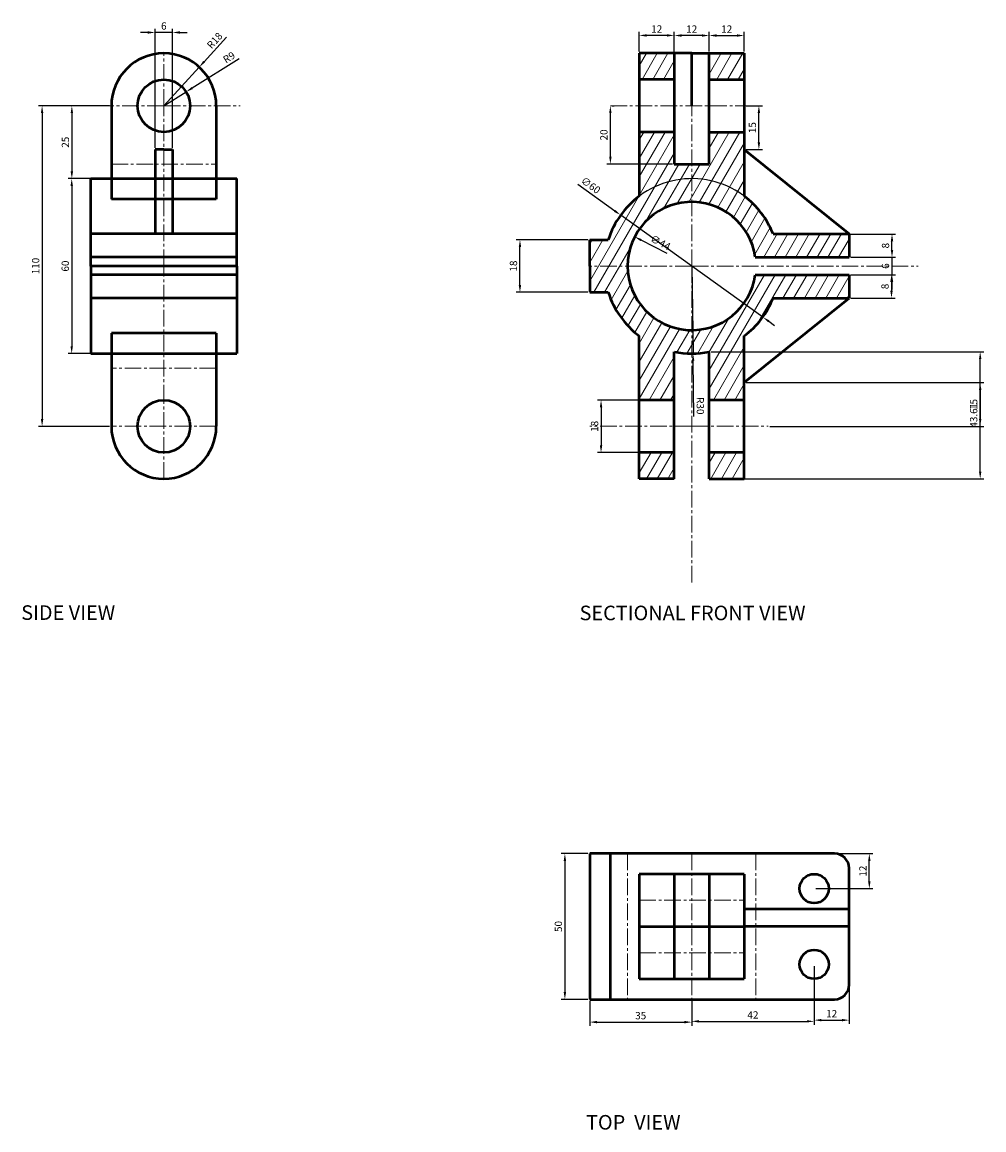
# Model space of a CAD drawing. Units: millimetres. Extents: x 2364 to 2785, y 1000 to 1694.
# Tile 1 of 2: x 2450 to 2780, y 1000 to 1380. Entities that reach past the tile are written whole.
import ezdxf

# ---------------------------------------------------------------- set-up
doc = ezdxf.new("R2010")
doc.units = ezdxf.units.MM
doc.linetypes.add('CENTER2', pattern=[28.575, 19.05, -3.175, 3.175, -3.175])
for name, color, linetype, lineweight in [('M-CNTR', 1, 'CENTER2', 18), ('M-DIMS', 2, 'Continuous', 25), ('M-HATC', 8, 'Continuous', 18), ('M-OUTL', 7, 'Continuous', 50), ('M-TEXT', 3, 'Continuous', 25)]:
    doc.layers.add(name, color=color, linetype=linetype, lineweight=lineweight)
doc.styles.get("Standard").update_dxf_attribs({"font": 'arial.ttf'})
doc.dimstyles.new('ISO-25', dxfattribs={"dimtxt": 2.5, "dimasz": 2.5, "dimexe": 1.25, "dimexo": 0.625, "dimtad": 1, "dimtxsty": 'Standard', "dimcen": 2.5, "dimadec": 0, "dimazin": 0, "dimtfac": 1, "dimtmove": 0, "dimatfit": 3, "dimfxl": 1, "dimarcsym": 0})

# ---------------------------------------------------------------- blocks, each defined once
blk = doc.blocks.new('*D17')
at = {"layer": 'Defpoints', "color": 0, "transparency": 16777216}
for p in [(2697.55, 1375.5), (2685.55, 1369.38), (2697.55, 1369.38)]:
    blk.add_point(p, dxfattribs=at)
at = {"layer": 'M-DIMS', "color": 0, "lineweight": -2, "transparency": 16777216}
for p, q in [((2685.55, 1370.01), (2685.55, 1376.75)), ((2697.55, 1370.01), (2697.55, 1376.75)), ((2688.05, 1375.5), (2695.05, 1375.5))]:
    blk.add_line(p, q, dxfattribs=at)
at = {"layer": 'M-DIMS', "color": 0, "transparency": 16777216}
for points in [[(2688.05, 1375.91), (2688.05, 1375.08), (2685.55, 1375.5)], [(2695.05, 1375.91), (2695.05, 1375.08), (2697.55, 1375.5)]]:
    blk.add_solid(points, dxfattribs=at)
at = {"layer": 'M-DIMS', "color": 0, "transparency": 16777216, "insert": (2691.55, 1377.38), "char_height": 2.5, "attachment_point": 5}
blk.add_mtext('12', dxfattribs=at)
blk = doc.blocks.new('*D18')
at = {"layer": 'Defpoints', "color": 0, "transparency": 16777216}
for p in [(2673.55, 1375.5), (2685.55, 1375.5), (2673.55, 1369.38)]:
    blk.add_point(p, dxfattribs=at)
at = {"layer": 'M-DIMS', "color": 0, "lineweight": -2, "transparency": 16777216}
for p, q in [((2673.55, 1370.01), (2673.55, 1376.75)), ((2685.55, 1376.12), (2685.55, 1376.75)), ((2683.05, 1375.5), (2676.05, 1375.5))]:
    blk.add_line(p, q, dxfattribs=at)
at = {"layer": 'M-DIMS', "color": 0, "transparency": 16777216}
for points in [[(2676.05, 1375.91), (2676.05, 1375.08), (2673.55, 1375.5)], [(2683.05, 1375.91), (2683.05, 1375.08), (2685.55, 1375.5)]]:
    blk.add_solid(points, dxfattribs=at)
at = {"layer": 'M-DIMS', "color": 0, "transparency": 16777216, "insert": (2679.55, 1377.38), "char_height": 2.5, "attachment_point": 5}
blk.add_mtext('12', dxfattribs=at)
blk = doc.blocks.new('*D19')
at = {"layer": 'Defpoints', "color": 0, "transparency": 16777216}
for p in [(2661.55, 1375.53), (2661.55, 1369.38), (2673.55, 1369.38)]:
    blk.add_point(p, dxfattribs=at)
at = {"layer": 'M-DIMS', "color": 0, "lineweight": -2, "transparency": 16777216}
for p, q in [((2661.55, 1370.01), (2661.55, 1376.78)), ((2673.55, 1370.01), (2673.55, 1376.78)), ((2671.05, 1375.53), (2664.05, 1375.53))]:
    blk.add_line(p, q, dxfattribs=at)
at = {"layer": 'M-DIMS', "color": 0, "transparency": 16777216}
for points in [[(2664.05, 1375.94), (2664.05, 1375.11), (2661.55, 1375.53)], [(2671.05, 1375.94), (2671.05, 1375.11), (2673.55, 1375.53)]]:
    blk.add_solid(points, dxfattribs=at)
at = {"layer": 'M-DIMS', "color": 0, "transparency": 16777216, "insert": (2667.55, 1377.41), "char_height": 2.5, "attachment_point": 5}
blk.add_mtext('12', dxfattribs=at)
blk = doc.blocks.new('*D20')
at = {"layer": 'Defpoints', "color": 0, "transparency": 16777216}
for p in [(2651.65, 1351.38), (2651.65, 1351.38), (2673.55, 1331.38)]:
    blk.add_point(p, dxfattribs=at)
at = {"layer": 'M-DIMS', "color": 0, "lineweight": -2, "transparency": 16777216}
for p, q in [((2652.27, 1351.38), (2652.9, 1351.38)), ((2651.65, 1333.88), (2651.65, 1348.88)), ((2672.93, 1331.38), (2650.4, 1331.38))]:
    blk.add_line(p, q, dxfattribs=at)
at = {"layer": 'M-DIMS', "color": 0, "transparency": 16777216}
for points in [[(2651.23, 1348.88), (2652.06, 1348.88), (2651.65, 1351.38)], [(2651.23, 1333.88), (2652.06, 1333.88), (2651.65, 1331.38)]]:
    blk.add_solid(points, dxfattribs=at)
at = {"layer": 'M-DIMS', "color": 0, "transparency": 16777216, "insert": (2649.74, 1341.38), "char_height": 2.5, "attachment_point": 5, "rotation": 90}
blk.add_mtext('20', dxfattribs=at)
blk = doc.blocks.new('*D21')
at = {"layer": 'Defpoints', "color": 0, "transparency": 16777216}
for p in [(2748.25, 1299.38), (2733.55, 1293.38), (2748.25, 1293.38)]:
    blk.add_point(p, dxfattribs=at)
at = {"layer": 'M-DIMS', "color": 0, "lineweight": -2, "transparency": 16777216}
for p, q in [((2748.25, 1301.88), (2748.25, 1304.38)), ((2748.25, 1299.38), (2748.25, 1293.38)), ((2748.88, 1299.38), (2749.5, 1299.38)), ((2734.18, 1293.38), (2749.5, 1293.38)), ((2748.25, 1290.88), (2748.25, 1288.38))]:
    blk.add_line(p, q, dxfattribs=at)
at = {"layer": 'M-DIMS', "color": 0, "transparency": 16777216}
for points in [[(2747.84, 1301.88), (2748.67, 1301.88), (2748.25, 1299.38)], [(2747.84, 1290.88), (2748.67, 1290.88), (2748.25, 1293.38)]]:
    blk.add_solid(points, dxfattribs=at)
at = {"layer": 'M-DIMS', "color": 0, "transparency": 16777216, "insert": (2746.35, 1296.38), "char_height": 2.5, "attachment_point": 5, "rotation": 90}
blk.add_mtext('6', dxfattribs=at)
blk = doc.blocks.new('*D22')
at = {"layer": 'Defpoints', "color": 0, "transparency": 16777216}
for p in [(2733.55, 1293.38), (2733.55, 1285.38), (2748.08, 1285.38)]:
    blk.add_point(p, dxfattribs=at)
at = {"layer": 'M-DIMS', "color": 0, "lineweight": -2, "transparency": 16777216}
for p, q in [((2734.18, 1293.38), (2749.33, 1293.38)), ((2748.08, 1290.88), (2748.08, 1287.88)), ((2734.18, 1285.38), (2749.33, 1285.38))]:
    blk.add_line(p, q, dxfattribs=at)
at = {"layer": 'M-DIMS', "color": 0, "transparency": 16777216}
for points in [[(2747.66, 1290.88), (2748.49, 1290.88), (2748.08, 1293.38)], [(2747.66, 1287.88), (2748.49, 1287.88), (2748.08, 1285.38)]]:
    blk.add_solid(points, dxfattribs=at)
at = {"layer": 'M-DIMS', "color": 0, "transparency": 16777216, "insert": (2746.18, 1289.38), "char_height": 2.5, "attachment_point": 5, "rotation": 90}
blk.add_mtext('8', dxfattribs=at)
blk = doc.blocks.new('*D23')
at = {"layer": 'Defpoints', "color": 0, "transparency": 16777216}
for p in [(2659.98, 1306.43), (2699.13, 1286.34)]:
    blk.add_point(p, dxfattribs=at)
at = {"layer": 'M-DIMS', "color": 0, "lineweight": -2, "transparency": 16777216}
blk.add_line((2671.14, 1300.7), (2662.2, 1305.29), dxfattribs=at)
at = {"layer": 'M-DIMS', "color": 0, "transparency": 16777216}
blk.add_solid([(2662.39, 1305.66), (2662.01, 1304.92), (2659.98, 1306.43)], dxfattribs=at)
at = {"layer": 'M-DIMS', "color": 0, "transparency": 16777216, "insert": (2668.68, 1304.18), "char_height": 2.5, "attachment_point": 5, "rotation": 332.8312}
blk.add_mtext('∅44', dxfattribs=at)
blk = doc.blocks.new('*D24')
at = {"layer": 'Defpoints', "color": 0, "transparency": 16777216}
for p in [(2655.18, 1313.88), (2703.92, 1278.89)]:
    blk.add_point(p, dxfattribs=at)
at = {"layer": 'M-DIMS', "color": 0, "lineweight": -2, "transparency": 16777216}
for p, q in [((2640.48, 1324.44), (2653.15, 1315.34)), ((2703.92, 1278.89), (2655.18, 1313.88)), ((2705.95, 1277.43), (2707.98, 1275.97))]:
    blk.add_line(p, q, dxfattribs=at)
blk.add_arc((2679.55, 1296.38), 30, 54.3238, 146.7095, dxfattribs=at)
at = {"layer": 'M-DIMS', "color": 0, "transparency": 16777216}
for points in [[(2653.4, 1315.68), (2652.91, 1315), (2655.18, 1313.88)], [(2706.2, 1277.77), (2705.71, 1277.09), (2703.92, 1278.89)]]:
    blk.add_solid(points, dxfattribs=at)
at = {"layer": 'M-DIMS', "color": 0, "transparency": 16777216, "insert": (2644.7, 1323.84), "char_height": 2.5, "attachment_point": 5, "rotation": 324.3222}
blk.add_mtext('∅60', dxfattribs=at)
blk = doc.blocks.new('*D25')
at = {"layer": 'Defpoints', "color": 0, "transparency": 16777216}
for p in [(2661.55, 1250.38), (2648.45, 1232.38), (2661.55, 1232.38)]:
    blk.add_point(p, dxfattribs=at)
at = {"layer": 'M-DIMS', "color": 0, "lineweight": -2, "transparency": 16777216}
for p, q in [((2660.93, 1250.38), (2647.2, 1250.38)), ((2648.45, 1247.88), (2648.45, 1234.88)), ((2660.93, 1232.38), (2647.2, 1232.38))]:
    blk.add_line(p, q, dxfattribs=at)
at = {"layer": 'M-DIMS', "color": 0, "transparency": 16777216}
for points in [[(2648.03, 1247.88), (2648.87, 1247.88), (2648.45, 1250.38)], [(2648.03, 1234.88), (2648.87, 1234.88), (2648.45, 1232.38)]]:
    blk.add_solid(points, dxfattribs=at)
at = {"layer": 'M-DIMS', "color": 0, "transparency": 16777216, "insert": (2646.55, 1241.38), "char_height": 2.5, "attachment_point": 5, "rotation": 90}
blk.add_mtext('18', dxfattribs=at)
blk = doc.blocks.new('*D26')
at = {"layer": 'Defpoints', "color": 0, "transparency": 16777216}
for p in [(2620.63, 1305.38), (2644.55, 1305.38), (2644.55, 1287.38)]:
    blk.add_point(p, dxfattribs=at)
at = {"layer": 'M-DIMS', "color": 0, "lineweight": -2, "transparency": 16777216}
for p, q in [((2643.93, 1305.38), (2619.38, 1305.38)), ((2620.63, 1289.88), (2620.63, 1302.88)), ((2643.93, 1287.38), (2619.38, 1287.38))]:
    blk.add_line(p, q, dxfattribs=at)
at = {"layer": 'M-DIMS', "color": 0, "transparency": 16777216}
for points in [[(2620.21, 1302.88), (2621.05, 1302.88), (2620.63, 1305.38)], [(2620.21, 1289.88), (2621.05, 1289.88), (2620.63, 1287.38)]]:
    blk.add_solid(points, dxfattribs=at)
at = {"layer": 'M-DIMS', "color": 0, "transparency": 16777216, "insert": (2618.73, 1296.38), "char_height": 2.5, "attachment_point": 5, "rotation": 90}
blk.add_mtext('18', dxfattribs=at)
blk = doc.blocks.new('*D27')
at = {"layer": 'Defpoints', "color": 0, "transparency": 16777216}
for p in [(2733.55, 1307.38), (2748.25, 1307.38), (2733.55, 1299.38)]:
    blk.add_point(p, dxfattribs=at)
at = {"layer": 'M-DIMS', "color": 0, "lineweight": -2, "transparency": 16777216}
for p, q in [((2734.18, 1307.38), (2749.5, 1307.38)), ((2748.25, 1301.88), (2748.25, 1304.88)), ((2734.18, 1299.38), (2749.5, 1299.38))]:
    blk.add_line(p, q, dxfattribs=at)
at = {"layer": 'M-DIMS', "color": 0, "transparency": 16777216}
for points in [[(2747.84, 1304.88), (2748.67, 1304.88), (2748.25, 1307.38)], [(2747.84, 1301.88), (2748.67, 1301.88), (2748.25, 1299.38)]]:
    blk.add_solid(points, dxfattribs=at)
at = {"layer": 'M-DIMS', "color": 0, "transparency": 16777216, "insert": (2746.35, 1303.38), "char_height": 2.5, "attachment_point": 5, "rotation": 90}
blk.add_mtext('8', dxfattribs=at)
blk = doc.blocks.new('*D28')
at = {"layer": 'Defpoints', "color": 0, "transparency": 16777216}
for p in [(2697.55, 1351.38), (2702.59, 1351.38), (2697.55, 1336.38)]:
    blk.add_point(p, dxfattribs=at)
at = {"layer": 'M-DIMS', "color": 0, "lineweight": -2, "transparency": 16777216}
for p, q in [((2698.18, 1351.38), (2703.84, 1351.38)), ((2702.59, 1338.88), (2702.59, 1348.88)), ((2698.18, 1336.38), (2703.84, 1336.38))]:
    blk.add_line(p, q, dxfattribs=at)
at = {"layer": 'M-DIMS', "color": 0, "transparency": 16777216}
for points in [[(2702.17, 1348.88), (2703.01, 1348.88), (2702.59, 1351.38)], [(2702.17, 1338.88), (2703.01, 1338.88), (2702.59, 1336.38)]]:
    blk.add_solid(points, dxfattribs=at)
at = {"layer": 'M-DIMS', "color": 0, "transparency": 16777216, "insert": (2700.69, 1343.88), "char_height": 2.5, "attachment_point": 5, "rotation": 90}
blk.add_mtext('15', dxfattribs=at)
blk = doc.blocks.new('*D29')
at = {"layer": 'Defpoints', "color": 0, "transparency": 16777216}
for p in [(2480.47, 1351.38), (2466.92, 1326.38), (2480.47, 1326.38)]:
    blk.add_point(p, dxfattribs=at)
at = {"layer": 'M-DIMS', "color": 0, "lineweight": -2, "transparency": 16777216}
for p, q in [((2479.84, 1351.38), (2465.67, 1351.38)), ((2466.92, 1348.88), (2466.92, 1328.88)), ((2479.84, 1326.38), (2465.67, 1326.38))]:
    blk.add_line(p, q, dxfattribs=at)
at = {"layer": 'M-DIMS', "color": 0, "transparency": 16777216}
for points in [[(2466.5, 1348.88), (2467.33, 1348.88), (2466.92, 1351.38)], [(2466.5, 1328.88), (2467.33, 1328.88), (2466.92, 1326.38)]]:
    blk.add_solid(points, dxfattribs=at)
at = {"layer": 'M-DIMS', "color": 0, "transparency": 16777216, "insert": (2465.02, 1338.88), "char_height": 2.5, "attachment_point": 5, "rotation": 90}
blk.add_mtext('25', dxfattribs=at)
blk = doc.blocks.new('*D30')
at = {"layer": 'Defpoints', "color": 0, "transparency": 16777216}
for p in [(2480.47, 1351.38), (2456.71, 1241.38), (2480.47, 1241.38)]:
    blk.add_point(p, dxfattribs=at)
at = {"layer": 'M-DIMS', "color": 0, "lineweight": -2, "transparency": 16777216}
for p, q in [((2479.84, 1351.38), (2455.46, 1351.38)), ((2456.71, 1348.88), (2456.71, 1243.88)), ((2479.84, 1241.38), (2455.46, 1241.38))]:
    blk.add_line(p, q, dxfattribs=at)
at = {"layer": 'M-DIMS', "color": 0, "transparency": 16777216}
for points in [[(2456.29, 1348.88), (2457.13, 1348.88), (2456.71, 1351.38)], [(2456.29, 1243.88), (2457.13, 1243.88), (2456.71, 1241.38)]]:
    blk.add_solid(points, dxfattribs=at)
at = {"layer": 'M-DIMS', "color": 0, "transparency": 16777216, "insert": (2454.81, 1296.38), "char_height": 2.5, "attachment_point": 5, "rotation": 90}
blk.add_mtext('110', dxfattribs=at)
blk = doc.blocks.new('*D31')
at = {"layer": 'Defpoints', "color": 0, "transparency": 16777216}
for p in [(2480.47, 1326.38), (2466.87, 1266.38), (2480.47, 1266.38)]:
    blk.add_point(p, dxfattribs=at)
at = {"layer": 'M-DIMS', "color": 0, "lineweight": -2, "transparency": 16777216}
for p, q in [((2479.84, 1326.38), (2465.62, 1326.38)), ((2466.87, 1323.88), (2466.87, 1268.88)), ((2479.84, 1266.38), (2465.62, 1266.38))]:
    blk.add_line(p, q, dxfattribs=at)
at = {"layer": 'M-DIMS', "color": 0, "transparency": 16777216}
for points in [[(2466.45, 1323.88), (2467.29, 1323.88), (2466.87, 1326.38)], [(2466.45, 1268.88), (2467.29, 1268.88), (2466.87, 1266.38)]]:
    blk.add_solid(points, dxfattribs=at)
at = {"layer": 'M-DIMS', "color": 0, "transparency": 16777216, "insert": (2464.97, 1296.38), "char_height": 2.5, "attachment_point": 5, "rotation": 90}
blk.add_mtext('60', dxfattribs=at)
blk = doc.blocks.new('*D32')
at = {"layer": 'Defpoints', "color": 0, "transparency": 16777216}
for p in [(2495.47, 1376.54), (2495.47, 1336.38), (2501.47, 1336.38)]:
    blk.add_point(p, dxfattribs=at)
at = {"layer": 'M-DIMS', "color": 0, "lineweight": -2, "transparency": 16777216}
for p, q in [((2492.97, 1376.54), (2490.47, 1376.54)), ((2495.47, 1337.01), (2495.47, 1377.79)), ((2501.47, 1376.54), (2495.47, 1376.54)), ((2501.47, 1337.01), (2501.47, 1377.79)), ((2503.97, 1376.54), (2506.47, 1376.54))]:
    blk.add_line(p, q, dxfattribs=at)
at = {"layer": 'M-DIMS', "color": 0, "transparency": 16777216}
for points in [[(2492.97, 1376.96), (2492.97, 1376.12), (2495.47, 1376.54)], [(2503.97, 1376.96), (2503.97, 1376.12), (2501.47, 1376.54)]]:
    blk.add_solid(points, dxfattribs=at)
at = {"layer": 'M-DIMS', "color": 0, "transparency": 16777216, "insert": (2498.47, 1378.44), "char_height": 2.5, "attachment_point": 5}
blk.add_mtext('6', dxfattribs=at)
blk = doc.blocks.new('*D33')
at = {"layer": 'Defpoints', "color": 0, "transparency": 16777216}
for p in [(2510.61, 1364.68), (2498.47, 1351.38)]:
    blk.add_point(p, dxfattribs=at)
at = {"layer": 'M-DIMS', "color": 0, "lineweight": -2, "transparency": 16777216}
for p, q in [((2519.99, 1374.95), (2512.29, 1366.52)), ((2498.47, 1351.38), (2510.61, 1364.68))]:
    blk.add_line(p, q, dxfattribs=at)
at = {"layer": 'M-DIMS', "color": 0, "transparency": 16777216}
blk.add_solid([(2511.99, 1366.8), (2512.6, 1366.24), (2510.61, 1364.68)], dxfattribs=at)
at = {"layer": 'M-DIMS', "color": 0, "transparency": 16777216, "insert": (2516.15, 1373.56), "char_height": 2.5, "attachment_point": 5, "rotation": 47.5926}
blk.add_mtext('R18', dxfattribs=at)
blk = doc.blocks.new('*D34')
at = {"layer": 'Defpoints', "color": 0, "transparency": 16777216}
for p in [(2506.1, 1356.16), (2498.47, 1351.38)]:
    blk.add_point(p, dxfattribs=at)
at = {"layer": 'M-DIMS', "color": 0, "lineweight": -2, "transparency": 16777216}
for p, q in [((2524.26, 1367.51), (2508.22, 1357.48)), ((2498.47, 1351.38), (2506.1, 1356.16))]:
    blk.add_line(p, q, dxfattribs=at)
at = {"layer": 'M-DIMS', "color": 0, "transparency": 16777216}
blk.add_solid([(2508, 1357.83), (2508.44, 1357.13), (2506.1, 1356.16)], dxfattribs=at)
at = {"layer": 'M-DIMS', "color": 0, "transparency": 16777216, "insert": (2521.01, 1367.72), "char_height": 2.5, "attachment_point": 5, "rotation": 32.0078}
blk.add_mtext('R9', dxfattribs=at)
blk = doc.blocks.new('*D35')
at = {"layer": 'Defpoints', "color": 0, "transparency": 16777216}
for p in [(2721.55, 1094.74), (2740.47, 1094.74), (2721.55, 1082.74)]:
    blk.add_point(p, dxfattribs=at)
at = {"layer": 'M-DIMS', "color": 0, "lineweight": -2, "transparency": 16777216}
for p, q in [((2722.18, 1094.74), (2741.72, 1094.74)), ((2740.47, 1085.24), (2740.47, 1092.24)), ((2722.18, 1082.74), (2741.72, 1082.74))]:
    blk.add_line(p, q, dxfattribs=at)
at = {"layer": 'M-DIMS', "color": 0, "transparency": 16777216}
for points in [[(2740.06, 1092.24), (2740.89, 1092.24), (2740.47, 1094.74)], [(2740.06, 1085.24), (2740.89, 1085.24), (2740.47, 1082.74)]]:
    blk.add_solid(points, dxfattribs=at)
at = {"layer": 'M-DIMS', "color": 0, "transparency": 16777216, "insert": (2738.59, 1088.74), "char_height": 2.5, "attachment_point": 5, "rotation": 90}
blk.add_mtext('12', dxfattribs=at)
blk = doc.blocks.new('*D36')
at = {"layer": 'Defpoints', "color": 0, "transparency": 16777216}
for p in [(2644.55, 1094.74), (2636.04, 1044.74), (2644.55, 1044.74)]:
    blk.add_point(p, dxfattribs=at)
at = {"layer": 'M-DIMS', "color": 0, "lineweight": -2, "transparency": 16777216}
for p, q in [((2643.93, 1094.74), (2634.79, 1094.74)), ((2636.04, 1092.24), (2636.04, 1047.24)), ((2643.93, 1044.74), (2634.79, 1044.74))]:
    blk.add_line(p, q, dxfattribs=at)
at = {"layer": 'M-DIMS', "color": 0, "transparency": 16777216}
for points in [[(2635.62, 1092.24), (2636.46, 1092.24), (2636.04, 1094.74)], [(2635.62, 1047.24), (2636.46, 1047.24), (2636.04, 1044.74)]]:
    blk.add_solid(points, dxfattribs=at)
at = {"layer": 'M-DIMS', "color": 0, "transparency": 16777216, "insert": (2634.14, 1069.74), "char_height": 2.5, "attachment_point": 5, "rotation": 90}
blk.add_mtext('50', dxfattribs=at)
blk = doc.blocks.new('*D37')
at = {"layer": 'Defpoints', "color": 0, "transparency": 16777216}
for p in [(2644.55, 1044.74), (2679.55, 1044.74), (2679.55, 1036.92)]:
    blk.add_point(p, dxfattribs=at)
at = {"layer": 'M-DIMS', "color": 0, "lineweight": -2, "transparency": 16777216}
for p, q in [((2644.55, 1044.12), (2644.55, 1035.67)), ((2679.55, 1044.12), (2679.55, 1035.67)), ((2647.05, 1036.92), (2677.05, 1036.92))]:
    blk.add_line(p, q, dxfattribs=at)
at = {"layer": 'M-DIMS', "color": 0, "transparency": 16777216}
for points in [[(2647.05, 1037.34), (2647.05, 1036.5), (2644.55, 1036.92)], [(2677.05, 1037.34), (2677.05, 1036.5), (2679.55, 1036.92)]]:
    blk.add_solid(points, dxfattribs=at)
at = {"layer": 'M-DIMS', "color": 0, "transparency": 16777216, "insert": (2662.05, 1038.82), "char_height": 2.5, "attachment_point": 5}
blk.add_mtext('35', dxfattribs=at)
blk = doc.blocks.new('*D38')
at = {"layer": 'Defpoints', "color": 0, "transparency": 16777216}
for p in [(2721.55, 1056.74), (2679.55, 1044.74), (2721.55, 1037.19)]:
    blk.add_point(p, dxfattribs=at)
at = {"layer": 'M-DIMS', "color": 0, "lineweight": -2, "transparency": 16777216}
for p, q in [((2721.55, 1056.12), (2721.55, 1035.94)), ((2679.55, 1044.12), (2679.55, 1035.94)), ((2682.05, 1037.19), (2719.05, 1037.19))]:
    blk.add_line(p, q, dxfattribs=at)
at = {"layer": 'M-DIMS', "color": 0, "transparency": 16777216}
for points in [[(2682.05, 1037.61), (2682.05, 1036.78), (2679.55, 1037.19)], [(2719.05, 1037.61), (2719.05, 1036.78), (2721.55, 1037.19)]]:
    blk.add_solid(points, dxfattribs=at)
at = {"layer": 'M-DIMS', "color": 0, "transparency": 16777216, "insert": (2700.55, 1039.07), "char_height": 2.5, "attachment_point": 5}
blk.add_mtext('42', dxfattribs=at)
blk = doc.blocks.new('*D39')
at = {"layer": 'Defpoints', "color": 0, "transparency": 16777216}
for p in [(2721.55, 1056.74), (2733.55, 1056.74), (2733.55, 1037.61)]:
    blk.add_point(p, dxfattribs=at)
at = {"layer": 'M-DIMS', "color": 0, "lineweight": -2, "transparency": 16777216}
for p, q in [((2721.55, 1056.12), (2721.55, 1036.36)), ((2733.55, 1056.12), (2733.55, 1036.36)), ((2724.05, 1037.61), (2731.05, 1037.61))]:
    blk.add_line(p, q, dxfattribs=at)
at = {"layer": 'M-DIMS', "color": 0, "transparency": 16777216}
for points in [[(2724.05, 1038.02), (2724.05, 1037.19), (2721.55, 1037.61)], [(2731.05, 1038.02), (2731.05, 1037.19), (2733.55, 1037.61)]]:
    blk.add_solid(points, dxfattribs=at)
at = {"layer": 'M-DIMS', "color": 0, "transparency": 16777216, "insert": (2727.55, 1039.49), "char_height": 2.5, "attachment_point": 5}
blk.add_mtext('12', dxfattribs=at)
blk = doc.blocks.new('*D40')
at = {"layer": 'Defpoints', "color": 0, "transparency": 16777216}
for p in [(2685.55, 1266.99), (2778.5, 1266.99), (2685.55, 1223.38)]:
    blk.add_point(p, dxfattribs=at)
at = {"layer": 'M-DIMS', "color": 0, "lineweight": -2, "transparency": 16777216}
for p, q in [((2686.18, 1266.99), (2779.75, 1266.99)), ((2778.5, 1225.88), (2778.5, 1264.49)), ((2686.18, 1223.38), (2779.75, 1223.38))]:
    blk.add_line(p, q, dxfattribs=at)
at = {"layer": 'M-DIMS', "color": 0, "transparency": 16777216}
for points in [[(2778.09, 1264.49), (2778.92, 1264.49), (2778.5, 1266.99)], [(2778.09, 1225.88), (2778.92, 1225.88), (2778.5, 1223.38)]]:
    blk.add_solid(points, dxfattribs=at)
at = {"layer": 'M-DIMS', "color": 0, "transparency": 16777216, "insert": (2776.6, 1245.19), "char_height": 2.5, "attachment_point": 5, "rotation": 90}
blk.add_mtext('43.61', dxfattribs=at)
blk = doc.blocks.new('*D41')
at = {"layer": 'Defpoints', "color": 0, "transparency": 16777216}
for p in [(2697.55, 1256.38), (2705.76, 1241.38), (2778.5, 1241.38)]:
    blk.add_point(p, dxfattribs=at)
at = {"layer": 'M-DIMS', "color": 0, "lineweight": -2, "transparency": 16777216}
for p, q in [((2698.18, 1256.38), (2779.75, 1256.38)), ((2778.5, 1253.88), (2778.5, 1243.88)), ((2706.39, 1241.38), (2779.75, 1241.38))]:
    blk.add_line(p, q, dxfattribs=at)
at = {"layer": 'M-DIMS', "color": 0, "transparency": 16777216}
for points in [[(2778.09, 1253.88), (2778.92, 1253.88), (2778.5, 1256.38)], [(2778.09, 1243.88), (2778.92, 1243.88), (2778.5, 1241.38)]]:
    blk.add_solid(points, dxfattribs=at)
at = {"layer": 'M-DIMS', "color": 0, "transparency": 16777216, "insert": (2776.6, 1248.88), "char_height": 2.5, "attachment_point": 5, "rotation": 90}
blk.add_mtext('15', dxfattribs=at)
blk = doc.blocks.new('*D42')
at = {"layer": 'Defpoints', "color": 0, "transparency": 16777216}
for p in [(2679.55, 1296.38), (2680, 1266.39)]:
    blk.add_point(p, dxfattribs=at)
at = {"layer": 'M-DIMS', "color": 0, "lineweight": -2, "transparency": 16777216}
for p, q in [((2679.55, 1296.38), (2680, 1266.39)), ((2680.32, 1244.78), (2680.04, 1263.89))]:
    blk.add_line(p, q, dxfattribs=at)
at = {"layer": 'M-DIMS', "color": 0, "transparency": 16777216}
blk.add_solid([(2680.45, 1263.89), (2679.62, 1263.88), (2680, 1266.39)], dxfattribs=at)
at = {"layer": 'M-DIMS', "color": 0, "transparency": 16777216, "insert": (2682.17, 1248.42), "char_height": 2.5, "attachment_point": 5, "rotation": 270.8551}
blk.add_mtext('R30', dxfattribs=at)

msp = doc.modelspace()

# ---------------------------------------------------------------- hatches: boundary and pattern name
at = {"layer": 'M-HATC'}
h = msp.add_hatch(dxfattribs=at)
h.set_pattern_fill('ANSI31', color=256, angle=15)
h.paths.add_polyline_path([(2679.552, 1331.385), (2673.552, 1331.385), (2673.552, 1342.385), (2661.552, 1342.385), (2661.552, 1320.385, 0.1569199), (2650.934, 1305.385), (2644.552, 1305.385), (2644.552, 1296.385), (2657.552, 1296.385, -0.4142136), (2679.552, 1318.385)])
h.paths.add_polyline_path([(2697.552, 1342.385), (2685.552, 1342.385), (2685.552, 1331.385), (2679.552, 1331.385), (2679.552, 1318.385, -0.3746932), (2701.347, 1299.385), (2733.552, 1299.385), (2733.552, 1307.385), (2707.463, 1307.385, 0.13885), (2697.552, 1320.385)])
h.paths.add_polyline_path([(2697.552, 1272.385, 0.13885), (2707.463, 1285.385), (2733.552, 1285.385), (2733.552, 1293.385), (2701.347, 1293.385, -0.3746932), (2679.552, 1274.385), (2679.552, 1266.385, 0.050382), (2685.552, 1266.991), (2685.552, 1250.385), (2697.552, 1250.385)])
h.paths.add_polyline_path([(2679.552, 1274.385, -0.4142136), (2657.552, 1296.385), (2644.552, 1296.385), (2644.552, 1287.385), (2650.934, 1287.385, 0.1569199), (2661.552, 1272.385), (2661.552, 1250.385), (2673.552, 1250.385), (2673.552, 1266.991, 0.050382), (2679.552, 1266.385)])
h.paths.add_polyline_path([(2673.552, 1232.385), (2661.552, 1232.385), (2661.552, 1223.385), (2673.552, 1223.385)])
h.paths.add_polyline_path([(2697.552, 1232.385), (2685.552, 1232.385), (2685.552, 1223.385), (2697.552, 1223.385)])
h.paths.add_polyline_path([(2673.552, 1369.385), (2661.552, 1369.385), (2661.552, 1360.385), (2673.552, 1360.385)])
h.paths.add_polyline_path([(2697.552, 1369.385), (2685.552, 1369.385), (2685.552, 1360.385), (2697.552, 1360.385)])

# ---------------------------------------------------------------- linework, layer by layer
at = {"layer": 'M-CNTR', "ltscale": 0.3}
for p, q in [((2498.468, 1351.385), (2498.468, 1369.385)), ((2498.468, 1351.385), (2471.755, 1351.385)), ((2498.468, 1296.385), (2498.468, 1351.385)), ((2498.468, 1351.385), (2524.69, 1351.385)), ((2651.646, 1351.385), (2703.004, 1351.385)), ((2679.552, 1296.385), (2679.552, 1351.385)), ((2480.468, 1331.385), (2516.468, 1331.385)), ((2523.468, 1296.385), (2473.468, 1296.385)), ((2498.468, 1249.902), (2498.468, 1296.385)), ((2679.552, 1296.385), (2644.552, 1296.385)), ((2679.552, 1296.385), (2757.254, 1296.385)), ((2679.552, 1296.385), (2679.552, 1187.563)), ((2516.468, 1261.385), (2480.468, 1261.385)), ((2498.468, 1223.385), (2498.468, 1249.902)), ((2516.468, 1241.385), (2480.468, 1241.385)), ((2679.552, 1241.385), (2644.552, 1241.385)), ((2679.552, 1241.385), (2705.762, 1241.385)), ((2657.552, 1094.744), (2657.552, 1044.744)), ((2679.552, 1094.744), (2679.552, 1044.744)), ((2701.552, 1094.744), (2701.552, 1044.744)), ((2661.552, 1078.744), (2697.552, 1078.744)), ((2661.552, 1060.744), (2697.552, 1060.744))]:
    msp.add_line(p, q, dxfattribs=at)
at = {"layer": 'M-OUTL'}
for p, q in [((2673.552, 1369.385), (2661.552, 1369.385)), ((2661.552, 1369.385), (2661.552, 1320.385)), ((2679.552, 1369.385), (2673.552, 1369.385)), ((2673.552, 1369.385), (2673.552, 1351.385)), ((2679.552, 1351.385), (2679.552, 1369.385)), ((2679.552, 1369.385), (2685.552, 1369.385)), ((2685.552, 1369.385), (2697.552, 1369.385)), ((2685.552, 1351.385), (2685.552, 1369.385)), ((2697.552, 1369.385), (2697.552, 1320.385)), ((2673.552, 1360.385), (2661.552, 1360.385)), ((2685.552, 1360.385), (2697.552, 1360.385)), ((2480.468, 1351.385), (2480.468, 1319.385)), ((2516.468, 1351.385), (2516.468, 1319.385)), ((2673.552, 1351.385), (2673.552, 1331.385)), ((2685.552, 1331.385), (2685.552, 1351.385)), ((2673.552, 1342.385), (2661.552, 1342.385)), ((2685.552, 1342.385), (2697.552, 1342.385)), ((2498.468, 1336.385), (2495.468, 1336.385)), ((2495.468, 1336.385), (2495.468, 1307.385)), ((2498.468, 1336.385), (2501.468, 1336.385)), ((2501.468, 1336.385), (2501.468, 1307.385)), ((2697.552, 1336.385), (2733.552, 1307.385)), ((2673.552, 1331.385), (2685.552, 1331.385)), ((2473.468, 1296.385), (2473.468, 1326.385)), ((2473.468, 1326.385), (2523.468, 1326.385)), ((2523.468, 1296.385), (2523.468, 1326.385)), ((2516.468, 1319.385), (2480.468, 1319.385)), ((2523.468, 1307.385), (2473.468, 1307.385)), ((2644.552, 1296.385), (2644.552, 1305.385)), ((2644.552, 1305.385), (2650.934, 1305.385)), ((2707.463, 1307.385), (2733.552, 1307.385)), ((2733.552, 1307.385), (2733.552, 1299.385)), ((2523.468, 1299.385), (2473.468, 1299.385)), ((2473.468, 1296.385), (2473.468, 1266.385)), ((2523.468, 1296.385), (2473.468, 1296.385)), ((2523.468, 1296.385), (2523.468, 1266.385)), ((2644.552, 1296.385), (2644.552, 1287.385)), ((2701.347, 1299.385), (2733.552, 1299.385)), ((2523.468, 1293.385), (2473.468, 1293.385)), ((2701.347, 1293.385), (2733.552, 1293.385)), ((2733.552, 1293.385), (2733.552, 1285.385)), ((2523.468, 1285.385), (2473.468, 1285.385)), ((2644.552, 1287.385), (2650.934, 1287.385)), ((2697.552, 1256.385), (2733.552, 1285.385)), ((2707.463, 1285.385), (2733.552, 1285.385)), ((2516.468, 1273.385), (2480.468, 1273.385)), ((2480.468, 1273.385), (2480.468, 1241.385)), ((2516.468, 1273.385), (2516.468, 1266.385)), ((2661.552, 1223.385), (2661.552, 1272.385)), ((2697.552, 1223.385), (2697.552, 1272.385)), ((2473.468, 1266.385), (2523.468, 1266.385)), ((2516.468, 1266.385), (2516.468, 1241.385)), ((2673.552, 1223.385), (2673.552, 1266.991)), ((2685.552, 1223.385), (2685.552, 1266.991)), ((2673.552, 1250.385), (2661.552, 1250.385)), ((2697.552, 1250.385), (2685.552, 1250.385)), ((2673.552, 1232.385), (2661.552, 1232.385)), ((2697.552, 1232.385), (2685.552, 1232.385)), ((2673.552, 1223.385), (2661.552, 1223.385)), ((2685.552, 1223.385), (2697.552, 1223.385)), ((2728.552, 1094.744), (2644.552, 1094.744)), ((2644.552, 1094.744), (2644.552, 1044.744)), ((2651.552, 1094.744), (2651.552, 1044.744)), ((2661.552, 1087.744), (2661.552, 1051.744)), ((2697.552, 1087.744), (2661.552, 1087.744)), ((2673.552, 1087.744), (2673.552, 1051.744)), ((2685.552, 1087.744), (2685.552, 1051.744)), ((2697.552, 1087.744), (2697.552, 1051.744)), ((2733.552, 1049.744), (2733.552, 1089.744)), ((2733.552, 1075.744), (2697.552, 1075.744)), ((2661.552, 1069.744), (2697.552, 1069.744)), ((2733.552, 1069.744), (2697.552, 1069.744)), ((2661.552, 1051.744), (2697.552, 1051.744)), ((2644.552, 1044.744), (2728.552, 1044.744))]:
    msp.add_line(p, q, dxfattribs=at)
for centre, radius in [((2498.468, 1351.385), 9), ((2498.468, 1241.385), 9), ((2721.552, 1082.744), 5), ((2721.552, 1056.744), 5)]:
    msp.add_circle(centre, radius, dxfattribs=at)
for centre, radius, start, end in [((2498.468, 1351.385), 18, 0, 180), ((2679.552, 1296.385), 30, 126.8699, 162.5424), ((2679.552, 1296.385), 30, 21.51019, 53.1301), ((2679.552, 1296.385), 22, 7.83748, 352.16252), ((2679.552, 1296.385), 30, 197.4576, 233.1301), ((2679.552, 1296.385), 30, 306.8699, 338.48981), ((2679.552, 1296.385), 30, 258.46304, 281.53696), ((2498.468, 1241.385), 18, 180, 0), ((2728.552, 1089.744), 5, 0, 90), ((2728.552, 1049.744), 5, 270, 0)]:
    msp.add_arc(centre, radius, start, end, dxfattribs=at)

# ---------------------------------------------------------------- texts
at = {"layer": 'M-TEXT', "char_height": 5, "attachment_point": 1}
for s, insert in [('SIDE VIEW', (2449.545, 1179.961)), ('SECTIONAL FRONT VIEW', (2641.072, 1179.837)), ('TOP  VIEW', (2643.285, 1005.045))]:
    msp.add_mtext_dynamic_manual_height_columns(s, width=88.56628, gutter_width=12.5, heights=[0], dxfattribs=dict(at, insert=insert))

# ---------------------------------------------------------------- dimensions: what is measured, and where the dimension line sits
at = {"layer": 'M-DIMS'}
for base, p1, p2, picture, middle in [((2495.468, 1376.54), (2501.468, 1336.385), (2495.468, 1336.385), '*D32', (2498.468, 1378.442)), ((2661.552, 1375.526), (2673.552, 1369.385), (2661.552, 1369.385), '*D19', (2667.552, 1377.406)), ((2673.552, 1375.496), (2685.552, 1375.496), (2673.552, 1369.385), '*D18', (2679.552, 1377.376)), ((2697.552, 1375.496), (2685.552, 1369.385), (2697.552, 1369.385), '*D17', (2691.552, 1377.376)), ((2721.552, 1037.195), (2679.552, 1044.744), (2721.552, 1056.744), '*D38', (2700.552, 1039.075)), ((2733.552, 1037.605), (2721.552, 1056.744), (2733.552, 1056.744), '*D39', (2727.552, 1039.485)), ((2679.552, 1036.921), (2644.552, 1044.744), (2679.552, 1044.744), '*D37', (2662.052, 1038.824))]:
    dim = msp.add_linear_dim(base=base, p1=p1, p2=p2, dimstyle='ISO-25', override={"dimclrd": 0, "dimclre": 0, "dimclrt": 0}, dxfattribs=at)
    dim.commit()
    dim.dimension.update_dxf_attribs({"geometry": picture, "text_midpoint": middle})
for center, mpoint, override, picture, middle in [((2498.468, 1351.385), (2510.607, 1364.676), {"dimclrd": 0, "dimclre": 0, "dimclrt": 0}, '*D33', (2517.554, 1372.282)), ((2498.468, 1351.385), (2506.099, 1356.155), {"dimclrd": 0, "dimclre": 0, "dimclrt": 0}, '*D34', (2522.02, 1366.107)), ((2679.552, 1296.385), (2680, 1266.388), {"dimdec": 0, "dimlfac": 1, "dimrnd": 0, "dimzin": 0, "dimdsep": 46, "dimlunit": 2}, '*D42', (2680.269, 1248.39))]:
    dim = msp.add_radius_dim(center=center, mpoint=mpoint, dimstyle='ISO-25', override=override, dxfattribs=at)
    dim.commit()
    dim.dimension.update_dxf_attribs({"geometry": picture, "text_midpoint": middle, "dimtype": 164})
for base, p1, p2, override, picture, middle in [((2456.712, 1241.385), (2480.468, 1351.385), (2480.468, 1241.385), {"dimclrd": 0, "dimclre": 0, "dimclrt": 0}, '*D30', (2454.81, 1296.385)), ((2466.916, 1326.385), (2480.468, 1351.385), (2480.468, 1326.385), {"dimclrd": 0, "dimclre": 0, "dimclrt": 0}, '*D29', (2465.015, 1338.885)), ((2651.646, 1351.385), (2673.552, 1331.385), (2651.646, 1351.385), {"dimclrd": 0, "dimclre": 0, "dimclrt": 0}, '*D20', (2649.744, 1341.385)), ((2702.591, 1351.385), (2697.552, 1336.385), (2697.552, 1351.385), {"dimclrd": 0, "dimclre": 0, "dimclrt": 0}, '*D28', (2700.69, 1343.885)), ((2466.871, 1266.385), (2480.468, 1326.385), (2480.468, 1266.385), {"dimclrd": 0, "dimclre": 0, "dimclrt": 0}, '*D31', (2464.97, 1296.385)), ((2620.631, 1305.385), (2644.552, 1287.385), (2644.552, 1305.385), {"dimclrd": 0, "dimclre": 0, "dimclrt": 0}, '*D26', (2618.729, 1296.385)), ((2748.254, 1307.385), (2733.552, 1299.385), (2733.552, 1307.385), {"dimclrd": 0, "dimclre": 0, "dimclrt": 0}, '*D27', (2746.352, 1303.385)), ((2748.254, 1293.385), (2748.254, 1299.385), (2733.552, 1293.385), {"dimclrd": 0, "dimclre": 0, "dimclrt": 0}, '*D21', (2746.352, 1296.385)), ((2748.078, 1285.385), (2733.552, 1293.385), (2733.552, 1285.385), {"dimclrd": 0, "dimclre": 0, "dimclrt": 0}, '*D22', (2746.176, 1289.385)), ((2778.504, 1266.991), (2685.552, 1223.385), (2685.552, 1266.991), {"dimdec": 2, "dimlfac": 1, "dimrnd": 0, "dimzin": 0, "dimdsep": 46, "dimlunit": 2}, '*D40', (2776.602, 1245.188)), ((2778.504, 1241.385), (2697.552, 1256.385), (2705.762, 1241.385), {"dimdec": 0, "dimlfac": 1, "dimrnd": 0, "dimzin": 0, "dimdsep": 46, "dimlunit": 2}, '*D41', (2776.603, 1248.885)), ((2648.45, 1232.385), (2661.552, 1250.385), (2661.552, 1232.385), {"dimclrd": 0, "dimclre": 0, "dimclrt": 0}, '*D25', (2646.548, 1241.385)), ((2636.041, 1044.744), (2644.552, 1094.744), (2644.552, 1044.744), {"dimclrd": 0, "dimclre": 0, "dimclrt": 0}, '*D36', (2634.14, 1069.744)), ((2740.474, 1094.744), (2721.552, 1082.744), (2721.552, 1094.744), {"dimclrd": 0, "dimclre": 0, "dimclrt": 0}, '*D35', (2738.594, 1088.744))]:
    dim = msp.add_linear_dim(base=base, p1=p1, p2=p2, angle=90, dimstyle='ISO-25', override=override, dxfattribs=at)
    dim.commit()
    dim.dimension.update_dxf_attribs({"geometry": picture, "text_midpoint": middle})
for p1, p2, picture, middle in [((2703.922, 1278.888), (2655.183, 1313.882), '*D24', (2643.548, 1322.236)), ((2699.125, 1286.339), (2659.98, 1306.43), '*D23', (2667.783, 1302.426))]:
    dim = msp.add_diameter_dim_2p(p1=p1, p2=p2, dimstyle='ISO-25', override={"dimclrd": 0, "dimclre": 0, "dimclrt": 0}, dxfattribs=at)
    dim.commit()
    dim.dimension.update_dxf_attribs({"geometry": picture, "text_midpoint": middle, "dimtype": 163})

doc.saveas('drawing.dxf')
